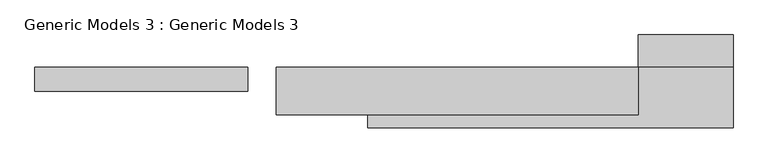
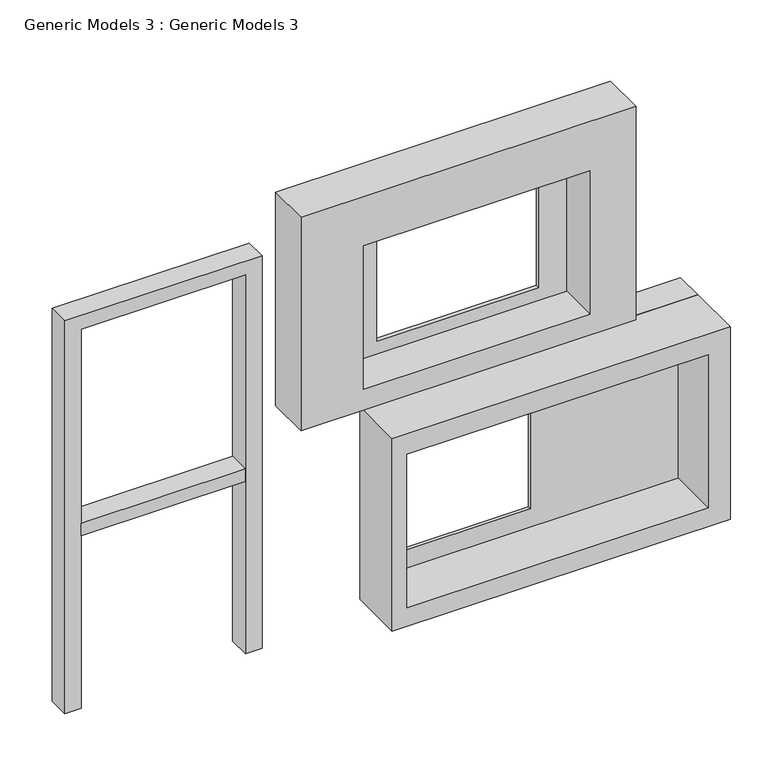
"""IFC4 building model written with IfcOpenShell, lengths in millimetres: proxy geometry, Generic Models 3 : Generic Models 3."""

from ifc_helpers import new_model, si_unit, frame, origin, origin_with_axes, place, context, project, spatial, polyline, outline, extrude, source, transform, mapped, element, save


def generic_models_3_generic_models_3_e29e7d65(model_context):
    return source(origin(), model_context, "Body", "SweptSolid", [
        extrude(outline(polyline([(-10799.9127168, -15164.946149), (-13085.9127168, -15164.946149), (-13085.9127168, -14860.146149), (-10799.9127168, -14860.146149), (-10799.9127168, -15164.946149)])), frame((0.0, 0.0, 2536.7442955), z_axis=(0.0, 0.0, 1.0), x_axis=(1.0, 0.0, 0.0)), (0.0, 0.0, 1.0), 185.7736016),
        extrude(outline(polyline([(0.0, -13314.5127168), (0.0, -13085.9127168), (5574.6202549, -13085.9127168), (5574.6202549, -10799.9127168), (0.0, -10799.9127168), (0.0, -10571.3127168), (5777.8202549, -10571.3127168), (5777.8202549, -13314.5127168), (0.0, -13314.5127168)])), frame((0.0, -15164.946149, 0.0), z_axis=(0.0, 1.0, 0.0), x_axis=(0.0, 0.0, 1.0)), (0.0, 0.0, 1.0), 304.8),
        extrude(outline(polyline([(537.8317429, -6685.1127168), (537.8317429, -8818.7127168), (270.5968393, -8818.7127168), (270.5968393, -4626.3601195), (2528.3677735, -4626.3601195), (2528.3677735, -6685.1127168), (537.8317429, -6685.1127168)])), frame((0.0, -14910.946149, 0.0), z_axis=(0.0, 1.0, 0.0), x_axis=(0.0, 0.0, 1.0)), (0.0, 0.0, 1.0), 50.8),
        extrude(outline(polyline([(0.0, -4322.4761094), (2829.1963889, -4322.4761094), (2829.1963889, -9027.8261094), (0.0, -9027.8261094), (0.0, -4322.4761094)]), holes=[polyline([(2528.3677735, -4626.3601195), (270.5968393, -4626.3601195), (270.5968393, -8818.7127168), (2528.3677735, -8818.7127168), (2528.3677735, -4626.3601195)])]), frame((0.0, -15636.6569663, 0.0), z_axis=(0.0, 1.0, 0.0), x_axis=(0.0, 0.0, 1.0)), (0.0, 0.0, 1.0), 776.5108173),
        extrude(outline(polyline([(-4322.4761094, -14860.146149), (-5541.6761094, -14860.146149), (-5541.6761094, -14441.6436399), (-4322.4761094, -14441.6436399), (-4322.4761094, -14860.146149)])), origin_with_axes(), (0.0, 0.0, 1.0), 2829.1963889),
        extrude(outline(polyline([(5677.6081175, -6176.6761094), (5677.6081175, -9333.3694007), (3564.6198177, -9333.3694007), (3564.6198177, -6176.6761094), (5677.6081175, -6176.6761094)]), holes=[polyline([(5311.3816242, -8818.7127168), (5311.3816242, -6570.3761094), (3754.5295223, -6570.3761094), (3754.5295223, -8818.7127168), (5311.3816242, -8818.7127168)])]), frame((0.0, -14910.946149, 0.0), z_axis=(0.0, 1.0, 0.0), x_axis=(0.0, 0.0, 1.0)), (0.0, 0.0, 1.0), 50.8),
        extrude(outline(polyline([(6400.8, -5541.6761094), (6400.8, -10203.7104375), (3259.8014539, -10203.7104375), (3259.8014539, -5541.6761094), (6400.8, -5541.6761094)]), holes=[polyline([(5677.6081175, -6176.6761094), (3564.6198177, -6176.6761094), (3564.6198177, -9333.3694007), (5677.6081175, -9333.3694007), (5677.6081175, -6176.6761094)])]), frame((0.0, -15469.746149, 0.0), z_axis=(0.0, 1.0, 0.0), x_axis=(0.0, 0.0, 1.0)), (0.0, 0.0, 1.0), 609.6),
    ])


if __name__ == "__main__":
    model = new_model("IFC4")
    model_context = context("Model", 3, world=origin())
    ifc_project = project(units=[si_unit("LENGTHUNIT", "METRE", prefix="MILLI")], contexts=[model_context])
    site = spatial("IfcSite", under=ifc_project)
    building = spatial("IfcBuilding", under=site)
    placement = place(None, origin())
    generic_models_3_generic_models_3_shape = generic_models_3_generic_models_3_e29e7d65(model_context)
    element("IfcBuildingElementProxy", 1, Name="Generic Models 3 : Generic Models 3", ObjectType="Generic Models 3 : Generic Models 3", at=placement, inside=building, context=model_context, shape_type="MappedRepresentation", body=[
        mapped(generic_models_3_generic_models_3_shape, transform((0.0, 0.0, 0.0), x_axis=(1.0, 0.0, 0.0), y_axis=(0.0, 1.0, 0.0), z_axis=(0.0, 0.0, 1.0))),
    ])
    save(model, "model.ifc")
